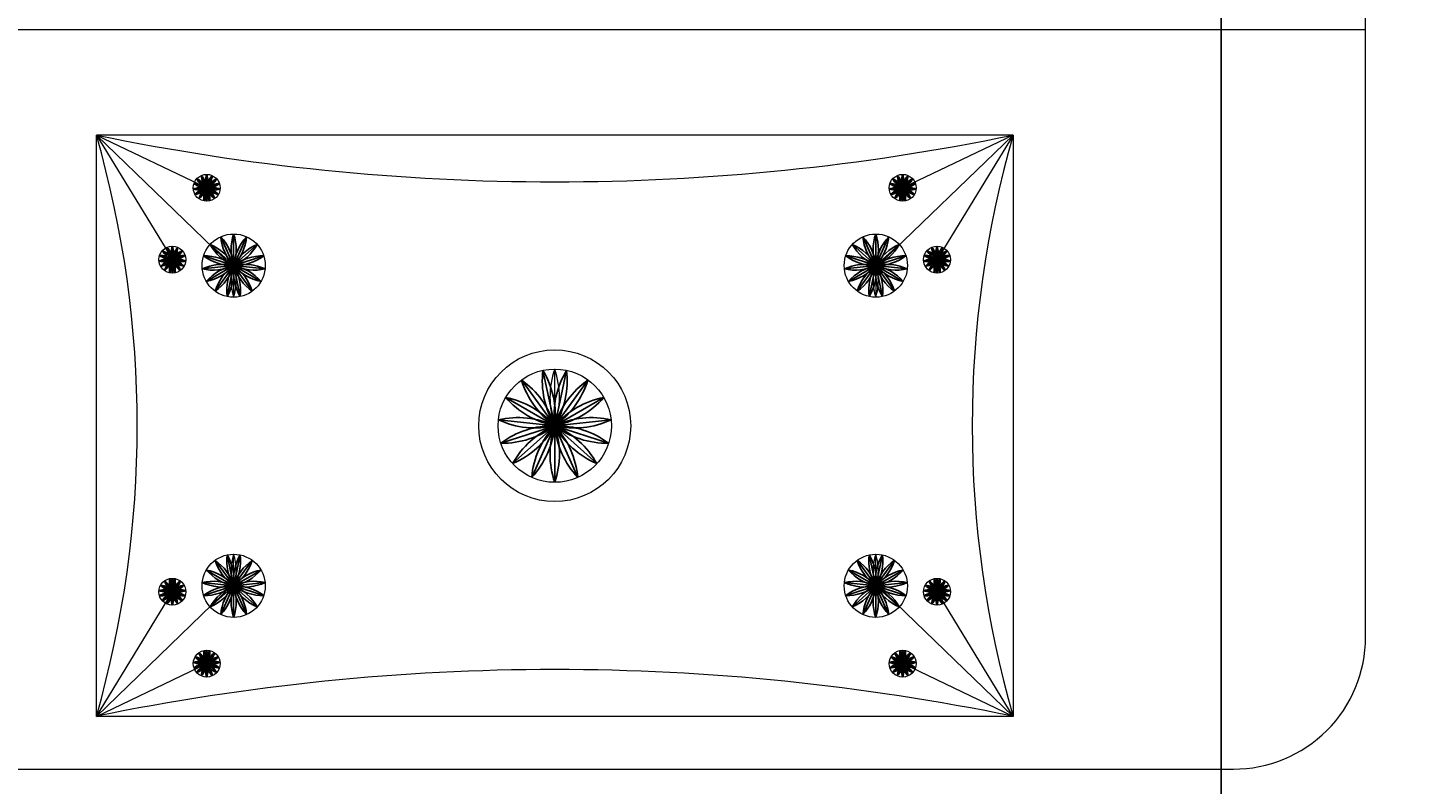
# Model space of a CAD drawing. Units: inches. Extents: x -61 to 1599, y -1316 to 257.
# Tile 50 of 204: x 149 to 185, y -428 to -408. Entities that reach past the tile are written whole.
import ezdxf

# ---------------------------------------------------------------- set-up
doc = ezdxf.new("R2010")
doc.units = ezdxf.units.IN
doc.header["$MEASUREMENT"] = 0
doc.layers.add('A-ANNO-DIMS', color=2, linetype='Continuous', lineweight=18)
doc.layers.add('FURNITURE', color=83, linetype='Continuous', lineweight=18)
doc.layers.add('LT', color=8, linetype='Continuous')
doc.styles.get("Standard").update_dxf_attribs({"font": 'arial.ttf'})
doc.dimstyles.get("Standard").update_dxf_attribs({"dimtxt": 0.18, "dimasz": 0.18, "dimexe": 0.18, "dimexo": 0.0625, "dimgap": 0.09, "dimtad": 0, "dimtih": 1, "dimtoh": 1, "dimdec": 0, "dimzin": 0, "dimdsep": 46, "dimlunit": 3, "dimtxsty": 'Standard', "dimcen": 0.09, "dimadec": 0, "dimazin": 0, "dimtfac": 1, "dimtdec": 0, "dimtofl": 0, "dimtmove": 0, "dimatfit": 3, "dimfxl": 1, "dimtolj": 1, "dimtzin": 0, "dimarcsym": 0})

# ---------------------------------------------------------------- blocks, each defined once
blk = doc.blocks.new('*U3')
at = {"layer": 'LT'}
blk.add_line((0, 0.175), (0, -0.175), dxfattribs=at)
for centre, start, end in [((0.509, 0), 160.9983, 199.0017), ((-0.509, 0), 340.9983, 19.0017)]:
    blk.add_arc(centre, 0.539, start, end, dxfattribs=at)
blk = doc.blocks.new('*U4')
at = {"layer": 'LT', "transparency": 16777216}
for p, rotation in [((-66.605, -18.692), 48.00000000000001), ((-66.546, -18.649), 24), ((-66.404, -18.649), 336.0000000000001), ((-66.345, -18.692), 312), ((-66.649, -18.828), 96), ((-66.642, -18.755), 72), ((-66.627, -18.897), 120), ((-66.578, -18.951), 144), ((-66.512, -18.981), 168.0000000000001), ((-66.439, -18.981), 192), ((-66.372, -18.951), 216), ((-66.323, -18.897), 240), ((-66.308, -18.755), 288.0000000000001), ((-66.301, -18.828), 264)]:
    blk.add_blockref('*U3', p, dxfattribs=dict(at, rotation=rotation))
blk.add_blockref('*U3', (-66.475, -18.634), dxfattribs=at)
blk = doc.blocks.new('*U20')
at = {"layer": 'LT'}
blk.add_line((0, 0.175), (0, -0.175), dxfattribs=at)
for centre, start, end in [((0.509, 0), 160.9983, 199.0017), ((-0.509, 0), 340.9983, 19.0017)]:
    blk.add_arc(centre, 0.539, start, end, dxfattribs=at)
blk = doc.blocks.new('*U21')
at = {"layer": 'LT', "transparency": 16777216}
for p, rotation in [((-66.605, -18.692), 48.00000000000001), ((-66.546, -18.649), 24), ((-66.404, -18.649), 336.0000000000001), ((-66.345, -18.692), 312), ((-66.649, -18.828), 96), ((-66.642, -18.755), 72), ((-66.627, -18.897), 120), ((-66.578, -18.951), 144), ((-66.512, -18.981), 168.0000000000001), ((-66.439, -18.981), 192), ((-66.372, -18.951), 216), ((-66.323, -18.897), 240), ((-66.308, -18.755), 288.0000000000001), ((-66.301, -18.828), 264)]:
    blk.add_blockref('*U20', p, dxfattribs=dict(at, rotation=rotation))
blk.add_blockref('*U20', (-66.475, -18.634), dxfattribs=at)
blk = doc.blocks.new('*U52')
at = {"layer": 'LT'}
blk.add_line((0, 0.175), (0, -0.175), dxfattribs=at)
for centre, start, end in [((0.509, 0), 160.9983, 199.0017), ((-0.509, 0), 340.9983, 19.0017)]:
    blk.add_arc(centre, 0.539, start, end, dxfattribs=at)
blk = doc.blocks.new('*U53')
at = {"layer": 'LT', "transparency": 16777216}
for p, rotation in [((-66.605, -18.692), 48.00000000000001), ((-66.546, -18.649), 24), ((-66.404, -18.649), 336.0000000000001), ((-66.345, -18.692), 312), ((-66.649, -18.828), 96), ((-66.642, -18.755), 72), ((-66.627, -18.897), 120), ((-66.578, -18.951), 144), ((-66.512, -18.981), 168.0000000000001), ((-66.439, -18.981), 192), ((-66.372, -18.951), 216), ((-66.323, -18.897), 240), ((-66.308, -18.755), 288.0000000000001), ((-66.301, -18.828), 264)]:
    blk.add_blockref('*U52', p, dxfattribs=dict(at, rotation=rotation))
blk.add_blockref('*U52', (-66.475, -18.634), dxfattribs=at)
blk = doc.blocks.new('*U29')
at = {"layer": 'LT'}
blk.add_line((0, 0.175), (0, -0.175), dxfattribs=at)
for centre, start, end in [((0.509, 0), 160.9983, 199.0017), ((-0.509, 0), 340.9983, 19.0017)]:
    blk.add_arc(centre, 0.539, start, end, dxfattribs=at)
blk = doc.blocks.new('*U30')
at = {"layer": 'LT', "transparency": 16777216}
for p, rotation in [((-66.605, -18.692), 48.00000000000001), ((-66.546, -18.649), 24), ((-66.404, -18.649), 336.0000000000001), ((-66.345, -18.692), 312), ((-66.649, -18.828), 96), ((-66.642, -18.755), 72), ((-66.627, -18.897), 120), ((-66.578, -18.951), 144), ((-66.512, -18.981), 168.0000000000001), ((-66.439, -18.981), 192), ((-66.372, -18.951), 216), ((-66.323, -18.897), 240), ((-66.308, -18.755), 288.0000000000001), ((-66.301, -18.828), 264)]:
    blk.add_blockref('*U29', p, dxfattribs=dict(at, rotation=rotation))
blk.add_blockref('*U29', (-66.475, -18.634), dxfattribs=at)
blk = doc.blocks.new('*U5')
at = {"layer": 'LT'}
blk.add_line((0, 0.412), (0, -0.412), dxfattribs=at)
for centre, start, end in [((1.198, 0), 160.9983, 199.0017), ((-1.198, 0), 340.9983, 19.0017)]:
    blk.add_arc(centre, 1.267, start, end, dxfattribs=at)
blk = doc.blocks.new('*U47')
at = {"layer": 'LT', "transparency": 16777216}
for p, rotation in [((-156.639, -43.959), 48.00000000000001), ((-156.501, -43.858), 24), ((-156.165, -43.858), 336.0000000000001), ((-156.027, -43.959), 312), ((-156.725, -44.108), 72), ((-155.941, -44.108), 288.0000000000001), ((-156.743, -44.278), 96), ((-156.69, -44.441), 120), ((-156.575, -44.569), 144), ((-156.419, -44.639), 168), ((-156.247, -44.639), 192), ((-156.091, -44.569), 216), ((-155.976, -44.441), 240), ((-155.923, -44.278), 264)]:
    blk.add_blockref('*U5', p, dxfattribs=dict(at, rotation=rotation))
blk.add_blockref('*U5', (-156.333, -43.823), dxfattribs=at)
blk = doc.blocks.new('*U22')
at = {"layer": 'LT'}
blk.add_line((0, 0.412), (0, -0.412), dxfattribs=at)
for centre, start, end in [((1.198, 0), 160.9983, 199.0017), ((-1.198, 0), 340.9983, 19.0017)]:
    blk.add_arc(centre, 1.267, start, end, dxfattribs=at)
blk = doc.blocks.new('*U23')
at = {"layer": 'LT', "transparency": 16777216}
for p, rotation in [((-156.639, -43.959), 48.00000000000001), ((-156.501, -43.858), 24), ((-156.165, -43.858), 336.0000000000001), ((-156.027, -43.959), 312), ((-156.725, -44.108), 72), ((-155.941, -44.108), 288.0000000000001), ((-156.743, -44.278), 96), ((-156.69, -44.441), 120), ((-156.575, -44.569), 144), ((-156.419, -44.639), 168), ((-156.247, -44.639), 192), ((-156.091, -44.569), 216), ((-155.976, -44.441), 240), ((-155.923, -44.278), 264)]:
    blk.add_blockref('*U22', p, dxfattribs=dict(at, rotation=rotation))
blk.add_blockref('*U22', (-156.333, -43.823), dxfattribs=at)
blk = doc.blocks.new('*U54')
at = {"layer": 'LT'}
blk.add_line((0, 0.739), (0, -0.739), dxfattribs=at)
for centre, start, end in [((2.147, 0), 160.9983, 199.0017), ((-2.147, 0), 340.9983, 19.0017)]:
    blk.add_arc(centre, 2.27, start, end, dxfattribs=at)
blk = doc.blocks.new('*U41')
at = {"layer": 'LT', "transparency": 16777216}
for p, rotation in [((-280.542, -78.621), 23.99999999999999), ((-279.941, -78.621), 336.0000000000001), ((-280.791, -78.801), 48.00000000000001), ((-279.692, -78.801), 312), ((-280.945, -79.067), 72), ((-279.539, -79.067), 288.0000000000001), ((-280.977, -79.373), 96), ((-280.882, -79.665), 120), ((-280.676, -79.894), 144), ((-280.395, -80.019), 168), ((-280.088, -80.019), 191.9999999999999), ((-279.807, -79.894), 216), ((-279.602, -79.665), 240), ((-279.507, -79.373), 264)]:
    blk.add_blockref('*U54', p, dxfattribs=dict(at, rotation=rotation))
blk.add_blockref('*U54', (-280.242, -78.557), dxfattribs=at)
blk = doc.blocks.new('*U42')
at = {"layer": 'LT'}
blk.add_line((0, 0.412), (0, -0.412), dxfattribs=at)
for centre, start, end in [((1.198, 0), 160.9983, 199.0017), ((-1.198, 0), 340.9983, 19.0017)]:
    blk.add_arc(centre, 1.267, start, end, dxfattribs=at)
blk = doc.blocks.new('*U43')
at = {"layer": 'LT', "transparency": 16777216}
for p, rotation in [((-156.639, -43.959), 48.00000000000001), ((-156.501, -43.858), 24), ((-156.165, -43.858), 336.0000000000001), ((-156.027, -43.959), 312), ((-156.725, -44.108), 72), ((-155.941, -44.108), 288.0000000000001), ((-156.743, -44.278), 96), ((-156.69, -44.441), 120), ((-156.575, -44.569), 144), ((-156.419, -44.639), 168), ((-156.247, -44.639), 192), ((-156.091, -44.569), 216), ((-155.976, -44.441), 240), ((-155.923, -44.278), 264)]:
    blk.add_blockref('*U42', p, dxfattribs=dict(at, rotation=rotation))
blk.add_blockref('*U42', (-156.333, -43.823), dxfattribs=at)
blk = doc.blocks.new('*U31')
at = {"layer": 'LT'}
blk.add_line((0, 0.412), (0, -0.412), dxfattribs=at)
for centre, start, end in [((1.198, 0), 160.9983, 199.0017), ((-1.198, 0), 340.9983, 19.0017)]:
    blk.add_arc(centre, 1.267, start, end, dxfattribs=at)
blk = doc.blocks.new('*U32')
at = {"layer": 'LT', "transparency": 16777216}
for p, rotation in [((-156.639, -43.959), 48.00000000000001), ((-156.501, -43.858), 24), ((-156.165, -43.858), 336.0000000000001), ((-156.027, -43.959), 312), ((-156.725, -44.108), 72), ((-155.941, -44.108), 288.0000000000001), ((-156.743, -44.278), 96), ((-156.69, -44.441), 120), ((-156.575, -44.569), 144), ((-156.419, -44.639), 168), ((-156.247, -44.639), 192), ((-156.091, -44.569), 216), ((-155.976, -44.441), 240), ((-155.923, -44.278), 264)]:
    blk.add_blockref('*U31', p, dxfattribs=dict(at, rotation=rotation))
blk.add_blockref('*U31', (-156.333, -43.823), dxfattribs=at)
blk = doc.blocks.new('*U48')
at = {"layer": 'LT'}
blk.add_line((0, 0.175), (0, -0.175), dxfattribs=at)
for centre, start, end in [((0.509, 0), 160.9983, 199.0017), ((-0.509, 0), 340.9983, 19.0017)]:
    blk.add_arc(centre, 0.539, start, end, dxfattribs=at)
blk = doc.blocks.new('*U49')
at = {"layer": 'LT', "transparency": 16777216}
for p, rotation in [((-66.605, -18.692), 48.00000000000001), ((-66.546, -18.649), 24), ((-66.404, -18.649), 336.0000000000001), ((-66.345, -18.692), 312), ((-66.649, -18.828), 96), ((-66.642, -18.755), 72), ((-66.627, -18.897), 120), ((-66.578, -18.951), 144), ((-66.512, -18.981), 168.0000000000001), ((-66.439, -18.981), 192), ((-66.372, -18.951), 216), ((-66.323, -18.897), 240), ((-66.308, -18.755), 288.0000000000001), ((-66.301, -18.828), 264)]:
    blk.add_blockref('*U48', p, dxfattribs=dict(at, rotation=rotation))
blk.add_blockref('*U48', (-66.475, -18.634), dxfattribs=at)
blk = doc.blocks.new('*U24')
at = {"layer": 'LT'}
blk.add_line((0, 0.175), (0, -0.175), dxfattribs=at)
for centre, start, end in [((0.509, 0), 160.9983, 199.0017), ((-0.509, 0), 340.9983, 19.0017)]:
    blk.add_arc(centre, 0.539, start, end, dxfattribs=at)
blk = doc.blocks.new('*U25')
at = {"layer": 'LT', "transparency": 16777216}
for p, rotation in [((-66.605, -18.692), 48.00000000000001), ((-66.546, -18.649), 24), ((-66.404, -18.649), 336.0000000000001), ((-66.345, -18.692), 312), ((-66.649, -18.828), 96), ((-66.642, -18.755), 72), ((-66.627, -18.897), 120), ((-66.578, -18.951), 144), ((-66.512, -18.981), 168.0000000000001), ((-66.439, -18.981), 192), ((-66.372, -18.951), 216), ((-66.323, -18.897), 240), ((-66.308, -18.755), 288.0000000000001), ((-66.301, -18.828), 264)]:
    blk.add_blockref('*U24', p, dxfattribs=dict(at, rotation=rotation))
blk.add_blockref('*U24', (-66.475, -18.634), dxfattribs=at)
blk = doc.blocks.new('*U50')
at = {"layer": 'LT'}
blk.add_line((0, 0.175), (0, -0.175), dxfattribs=at)
for centre, start, end in [((0.509, 0), 160.9983, 199.0017), ((-0.509, 0), 340.9983, 19.0017)]:
    blk.add_arc(centre, 0.539, start, end, dxfattribs=at)
blk = doc.blocks.new('*U51')
at = {"layer": 'LT', "transparency": 16777216}
for p, rotation in [((-66.605, -18.692), 48.00000000000001), ((-66.546, -18.649), 24), ((-66.404, -18.649), 336.0000000000001), ((-66.345, -18.692), 312), ((-66.649, -18.828), 96), ((-66.642, -18.755), 72), ((-66.627, -18.897), 120), ((-66.578, -18.951), 144), ((-66.512, -18.981), 168.0000000000001), ((-66.439, -18.981), 192), ((-66.372, -18.951), 216), ((-66.323, -18.897), 240), ((-66.308, -18.755), 288.0000000000001), ((-66.301, -18.828), 264)]:
    blk.add_blockref('*U50', p, dxfattribs=dict(at, rotation=rotation))
blk.add_blockref('*U50', (-66.475, -18.634), dxfattribs=at)
blk = doc.blocks.new('*U26')
at = {"layer": 'LT'}
blk.add_line((0, 0.175), (0, -0.175), dxfattribs=at)
for centre, start, end in [((0.509, 0), 160.9983, 199.0017), ((-0.509, 0), 340.9983, 19.0017)]:
    blk.add_arc(centre, 0.539, start, end, dxfattribs=at)
blk = doc.blocks.new('*U27')
at = {"layer": 'LT', "transparency": 16777216}
for p, rotation in [((-66.605, -18.692), 48.00000000000001), ((-66.546, -18.649), 24), ((-66.404, -18.649), 336.0000000000001), ((-66.345, -18.692), 312), ((-66.649, -18.828), 96), ((-66.642, -18.755), 72), ((-66.627, -18.897), 120), ((-66.578, -18.951), 144), ((-66.512, -18.981), 168.0000000000001), ((-66.439, -18.981), 192), ((-66.372, -18.951), 216), ((-66.323, -18.897), 240), ((-66.308, -18.755), 288.0000000000001), ((-66.301, -18.828), 264)]:
    blk.add_blockref('*U26', p, dxfattribs=dict(at, rotation=rotation))
blk.add_blockref('*U26', (-66.475, -18.634), dxfattribs=at)
blk = doc.blocks.new('BED-DOUBLE')
for p, q in [((1.272, 19.317), (70.263, 19.317)), ((37.147, 1.379), (37.147, 16.557)), ((61.064, 16.557), (37.147, 16.557)), ((37.147, 16.557), (40.027, 15.18)), ((37.147, 16.557), (40.715, 13.107)), ((37.147, 16.557), (39.13, 13.305)), ((61.064, 16.557), (57.496, 13.107)), ((61.064, 16.557), (58.185, 15.18)), ((61.064, 16.557), (59.081, 13.305)), ((40.027, 15.18), (40.027, 14.829)), ((58.185, 15.18), (58.185, 14.829)), ((39.13, 13.305), (39.13, 12.955)), ((40.729, 13.149), (40.729, 12.324)), ((57.483, 13.149), (57.483, 12.324)), ((59.081, 13.305), (59.081, 12.955)), ((49.106, 8.968), (49.106, 10.447)), ((40.729, 4.788), (40.729, 5.613)), ((57.483, 4.788), (57.483, 5.613)), ((37.147, 1.379), (40.715, 4.83)), ((39.13, 4.631), (39.13, 4.982)), ((61.064, 1.379), (57.496, 4.83)), ((59.081, 4.631), (59.081, 4.982)), ((37.147, 1.379), (39.13, 4.631)), ((61.064, 1.379), (59.081, 4.631)), ((40.027, 2.756), (40.027, 3.107)), ((58.185, 2.756), (58.185, 3.107)), ((37.147, 1.379), (40.027, 2.756)), ((61.064, 1.379), (58.185, 2.756)), ((61.064, 1.379), (61.064, 1.379))]:
    blk.add_line(p, q)
for points in [[(1.272, 88.537), (1.272, 3.449, 0.414214), (4.722, 0), (66.813, 0, 0.414214), (70.263, 3.449), (70.263, 88.537, 0.414214), (66.813, 91.987), (4.722, 91.987, 0.414214)], [(40.027, 15.18, 0.167358), (40.027, 14.829, 0.167358)], [(39.13, 13.305, 0.167358), (39.13, 12.955, 0.167358)], [(40.729, 13.149, 0.167358), (40.729, 12.324, 0.167358)], [(57.483, 12.324, 0.167358), (57.483, 13.149, 0.167358)], [(59.081, 12.955, 0.167358), (59.081, 13.305, 0.167358)], [(49.106, 8.968, 0.167358), (49.106, 10.447, 0.167358)], [(40.729, 5.613, 0.167358), (40.729, 4.788, 0.167358)], [(57.483, 4.788, 0.167358), (57.483, 5.613, 0.167358)], [(39.13, 4.982, 0.167358), (39.13, 4.631, 0.167358)], [(59.081, 4.631, 0.167358), (59.081, 4.982, 0.167358)], [(40.027, 3.107, 0.167358), (40.027, 2.756, 0.167358)], [(58.185, 2.756, 0.167358), (58.185, 3.107, 0.167358)]]:
    blk.add_lwpolyline(points, format="xyb", close=True)
blk.add_lwpolyline([(61.064, 16.557), (61.064, 1.379), (37.147, 1.379)])
for centre, radius in [((40.027, 15.18), 0.351), ((58.185, 15.18), 0.351), ((40.729, 13.149), 0.825), ((57.483, 13.149), 0.825), ((39.13, 13.305), 0.351), ((59.081, 13.305), 0.351), ((49.106, 8.968), 1.982), ((49.106, 8.968), 1.478), ((40.729, 4.788), 0.825), ((57.483, 4.788), 0.825), ((39.13, 4.631), 0.351), ((59.081, 4.631), 0.351), ((40.027, 2.756), 0.351), ((58.185, 2.756), 0.351)]:
    blk.add_circle(centre, radius)
for centre, radius, start, end in [((10.674, 8.968), 27.54, 344.0046, 15.9954), ((49.106, 74.54), 59.203, 258.34678, 281.65322), ((87.538, 8.968), 27.54, 164.0046, 195.9954), ((58.694, 15.005), 0.539, 160.9983, 199.0017), ((57.675, 15.005), 0.539, 340.9983, 19.0017), ((49.106, -56.603), 59.203, 78.34678, 101.65322)]:
    blk.add_arc(centre, radius, start, end)
for name, p in [('*U30', (106.502, 33.99)), ('*U23', (197.062, 57.384)), ('*U21', (105.605, 32.115))]:
    blk.add_blockref(name, p)
at = {"extrusion": (0, 0, -1), "zscale": -1}
for name, p in [('*U25', (8.291, 33.99)), ('*U32', (98.85, 57.384)), ('*U27', (7.394, 32.115))]:
    blk.add_blockref(name, p, dxfattribs=at)
at = {"rotation": 180}
for name, p in [('*U41', (-231.136, -70.328)), ('*U43', (-98.85, -39.447)), ('*U51', (-7.394, -14.178)), ('*U49', (-8.291, -16.053))]:
    blk.add_blockref(name, p, dxfattribs=at)
at = {"extrusion": (0, 0, -1), "zscale": -1, "rotation": 180}
for name, p in [('*U47', (-197.062, -39.447)), ('*U4', (-105.605, -14.178)), ('*U53', (-106.502, -16.053))]:
    blk.add_blockref(name, p, dxfattribs=at)
blk = doc.blocks.new('*D687')
at = {"layer": 'A-ANNO-DIMS', "color": 0, "lineweight": -2, "transparency": 16777216}
for p, q in [((289.418, 181.677), (-61.077, 181.677)), ((-60.897, 181.497), (-60.897, -528.952)), ((-60.897, -1239.765), (-60.897, -529.316)), ((319.64, -1239.945), (-61.077, -1239.945))]:
    blk.add_line(p, q, dxfattribs=at)
at = {"layer": 'A-ANNO-DIMS', "color": 0, "transparency": 16777216}
for points in [[(-60.927, 181.497), (-60.867, 181.497), (-60.897, 181.677)], [(-60.927, -1239.765), (-60.867, -1239.765), (-60.897, -1239.945)]]:
    blk.add_solid(points, dxfattribs=at)
at = {"layer": 'DEFPOINTS', "color": 0, "transparency": 16777216}
for p in [(289.481, 181.677), (-60.897, -1239.945), (319.703, -1239.945)]:
    blk.add_point(p, dxfattribs=at)
at = {"layer": 'A-ANNO-DIMS', "color": 0, "transparency": 16777216, "insert": (-60.897, -529.134), "char_height": 0.18, "attachment_point": 5}
blk.add_mtext('\\A1;1421.6', dxfattribs=at)
blk = doc.blocks.new('*D699')
at = {"layer": 'A-ANNO-DIMS', "color": 0, "lineweight": -2, "transparency": 16777216}
for p, q in [((835.64, -167.169), (-61.077, -167.169)), ((-60.897, -167.349), (-60.897, -306.726)), ((-60.897, -446.466), (-60.897, -307.09)), ((841.64, -446.646), (-61.077, -446.646))]:
    blk.add_line(p, q, dxfattribs=at)
at = {"layer": 'A-ANNO-DIMS', "color": 0, "transparency": 16777216}
for points in [[(-60.927, -167.349), (-60.867, -167.349), (-60.897, -167.169)], [(-60.927, -446.466), (-60.867, -446.466), (-60.897, -446.646)]]:
    blk.add_solid(points, dxfattribs=at)
at = {"layer": 'DEFPOINTS', "color": 0, "transparency": 16777216}
for p in [(835.703, -167.169), (-60.897, -446.646), (841.703, -446.646)]:
    blk.add_point(p, dxfattribs=at)
at = {"layer": 'A-ANNO-DIMS', "color": 0, "transparency": 16777216, "insert": (-60.897, -306.908), "char_height": 0.18, "attachment_point": 5}
blk.add_mtext('\\A1;279.5', dxfattribs=at)
blk = doc.blocks.new('*D700')
at = {"layer": 'A-ANNO-DIMS', "color": 0, "lineweight": -2, "transparency": 16777216}
for p, q in [((14.703, -616.882), (14.703, 257.457)), ((14.883, 257.277), (96.772, 257.277)), ((179.572, 257.277), (97.683, 257.277)), ((179.752, -616.882), (179.752, 257.457))]:
    blk.add_line(p, q, dxfattribs=at)
at = {"layer": 'A-ANNO-DIMS', "color": 0, "transparency": 16777216}
for points in [[(14.883, 257.307), (14.883, 257.247), (14.703, 257.277)], [(179.572, 257.307), (179.572, 257.247), (179.752, 257.277)]]:
    blk.add_solid(points, dxfattribs=at)
at = {"layer": 'DEFPOINTS', "color": 0, "transparency": 16777216}
for p in [(179.752, 257.277), (14.703, -616.945), (179.752, -616.945)]:
    blk.add_point(p, dxfattribs=at)
at = {"layer": 'A-ANNO-DIMS', "color": 0, "transparency": 16777216, "insert": (97.227, 257.277), "char_height": 0.18, "attachment_point": 5}
blk.add_mtext('\\A1;165.05', dxfattribs=at)

msp = doc.modelspace()

# ---------------------------------------------------------------- block references
at = {"layer": 'FURNITURE'}
msp.add_blockref('BED-DOUBLE', (113.2612, -427.6961), dxfattribs=at)

# ---------------------------------------------------------------- dimensions: what is measured, and where the dimension line sits
at = {"layer": 'A-ANNO-DIMS'}
dim = msp.add_linear_dim(base=(179.7521, 257.2771), p1=(14.7028, -616.9446), p2=(179.7521, -616.9446), dimstyle='Standard', override={"dimdec": 2, "dimlfac": 1, "dimrnd": 0, "dimzin": 0, "dimdsep": 46, "dimlunit": 2}, dxfattribs=at)
dim.commit()
dim.dimension.update_dxf_attribs({"geometry": '*D700', "text_midpoint": (97.2274, 257.2771)})
for base, p1, p2, picture, middle in [((-60.8972, -1239.9446), (289.4807, 181.6771), (319.7028, -1239.9446), '*D687', (-60.8972, -529.1337)), ((-60.8972, -446.6462), (835.7028, -167.169), (841.7028, -446.6462), '*D699', (-60.8972, -306.9076))]:
    dim = msp.add_linear_dim(base=base, p1=p1, p2=p2, angle=90, dimstyle='Standard', override={"dimdec": 1, "dimlfac": 1, "dimrnd": 0, "dimzin": 0, "dimdsep": 46, "dimlunit": 2}, dxfattribs=at)
    dim.commit()
    dim.dimension.update_dxf_attribs({"geometry": picture, "text_midpoint": middle})

doc.saveas('drawing.dxf')
